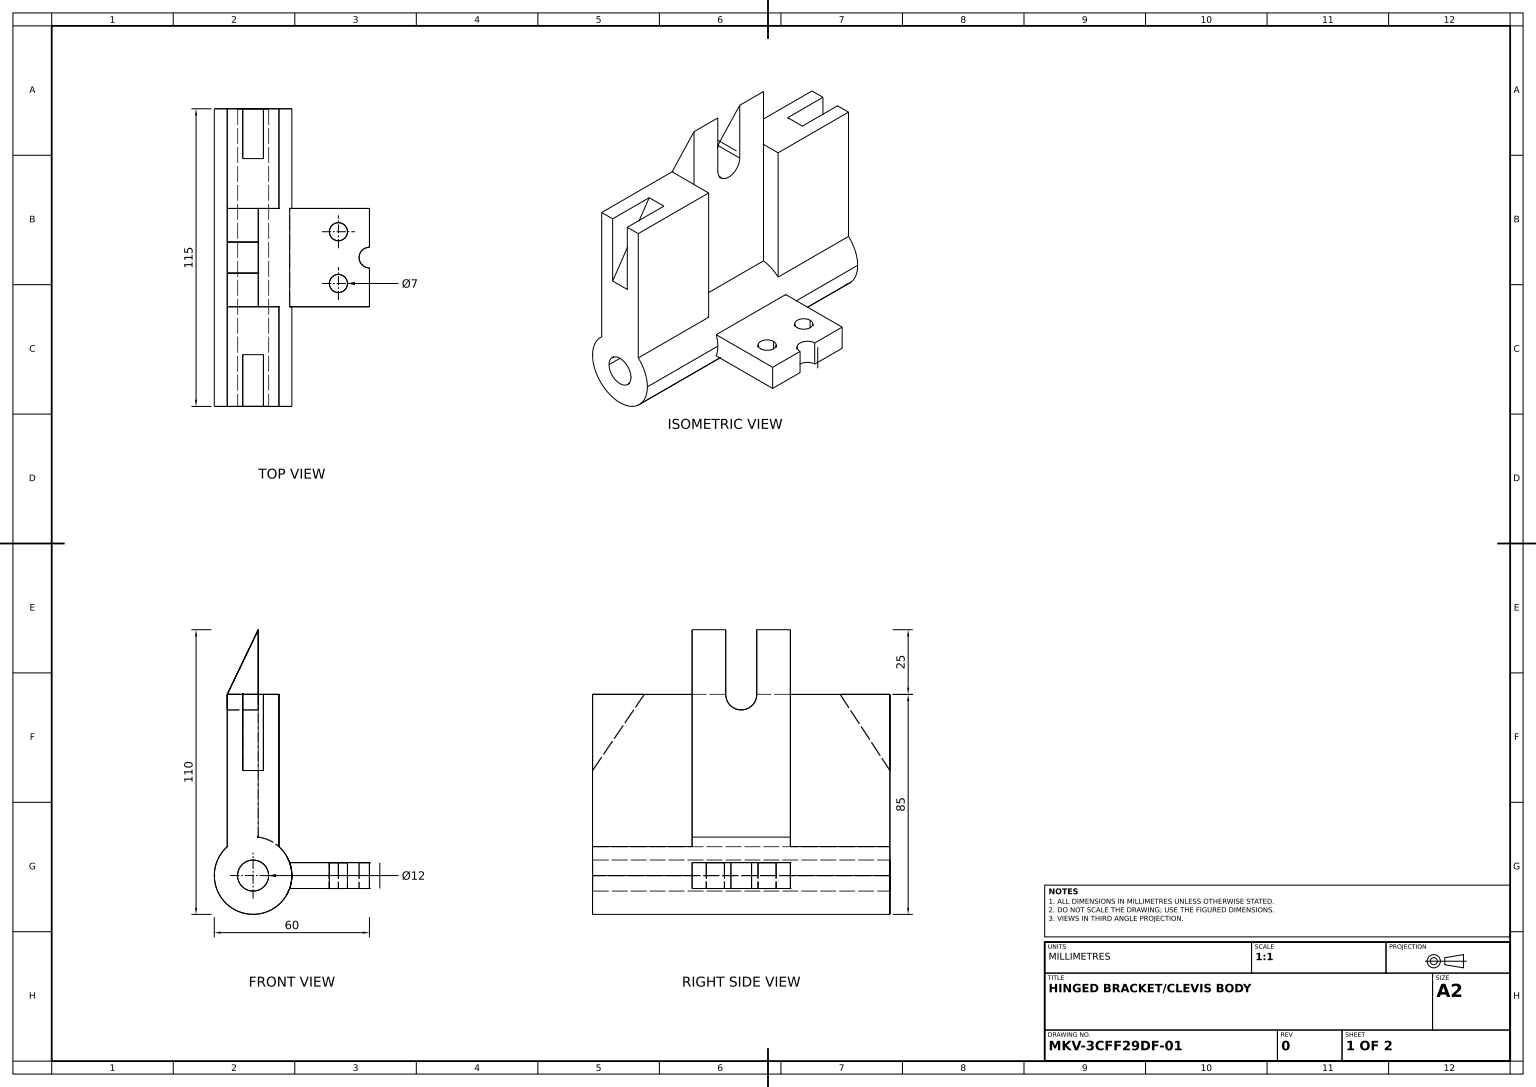
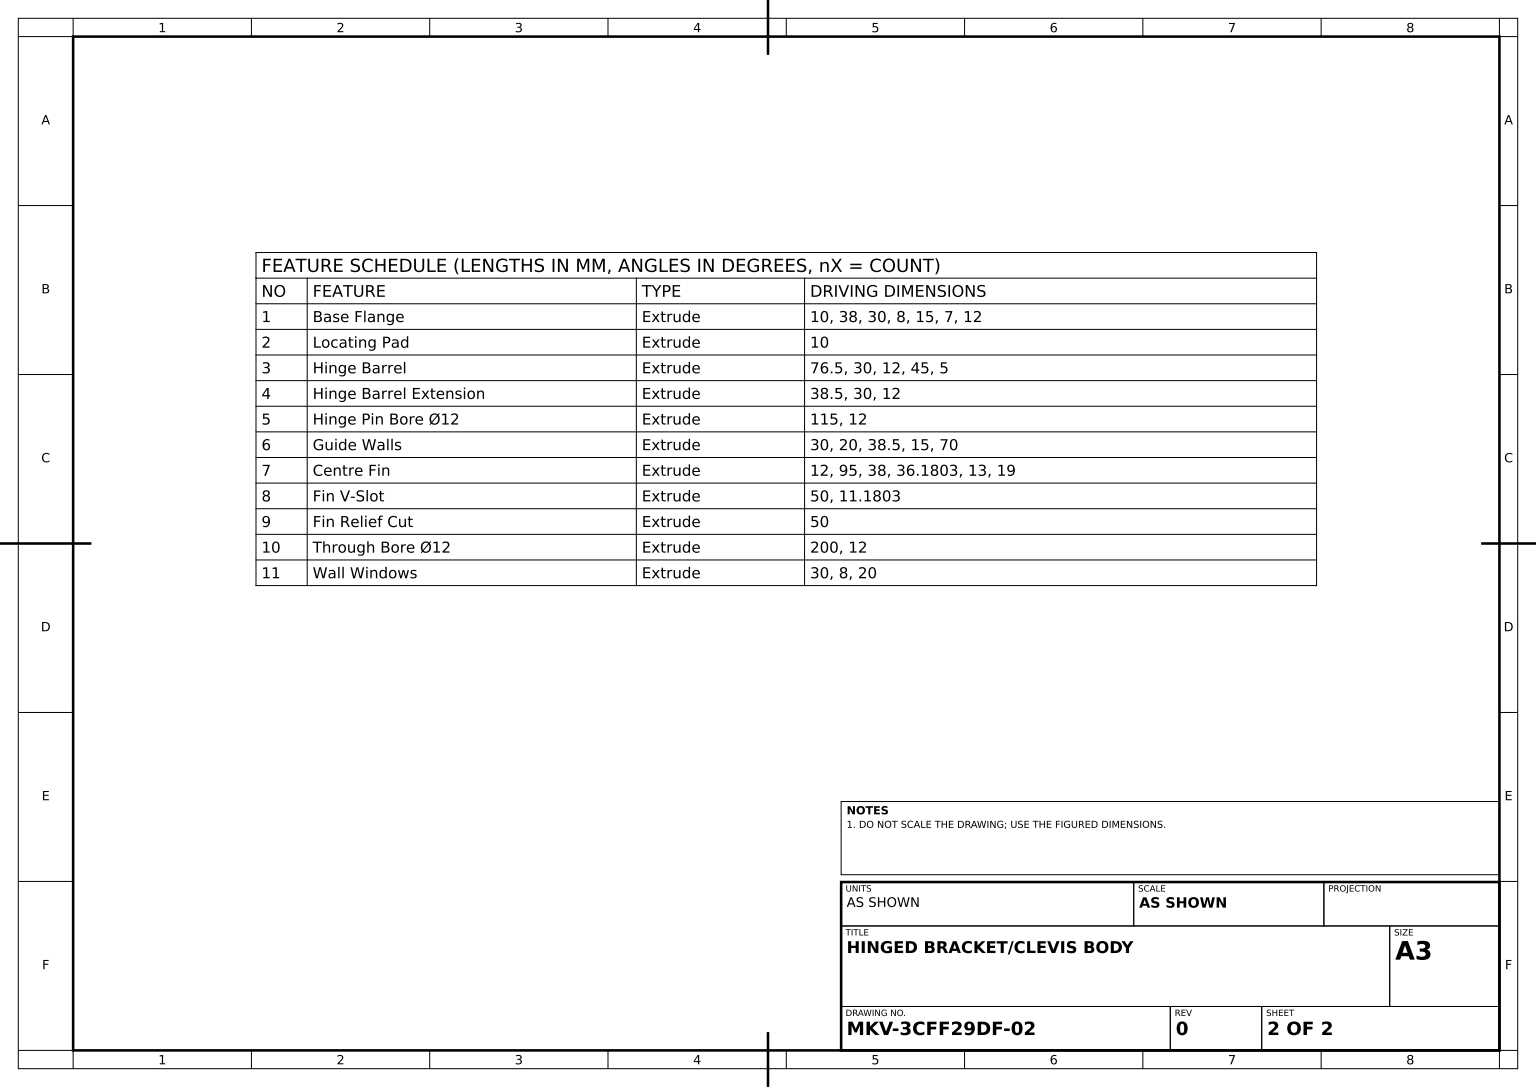
SolidWorks part; units mm, degrees
material "Plain Carbon Steel"
ref_plane "Front Plane" through (0, 0, 0) normal (0, 0, 1) x (1, 0, 0)
ref_plane "Top Plane" through (0, 0, 0) normal (0, 1, 0) x (1, 0, 0)
ref_plane "Right Plane" through (0, 0, 0) normal (1, 0, 0) x (0, 0, -1)
sketch "Base Flange Sketch" plane through (0, 0, 0) normal (0, 1, 0) x (1, 0, 0)
  line L0 (15, -4) -> (15, -19)
  line L1 (-15, 19) -> (15, 19)
  line L2 (-15, 19) -> (-15, -19)
  line L3 (-15, -19) -> (15, -19)
  line L4 (15, 19) -> (15, 4)
  line L5 (-15, 19) -> (15, -19) construction
  line L6 (-15, -19) -> (15, 19) construction
  arc A0 (15, 4) -> (15, -4) centre (15, 0) ccw
  circle A1 centre (3, 10) radius 3.5
  circle A2 centre (3, -10) radius 3.5
  point P0 (0, 0)
  dimension "D3" = 8
  dimension "D6" = 7
  dimension "D7" = 7
  dimension "D1" = 38
  dimension "D2" = 30
  dimension "D4" = 15
  dimension "D5" = 15
  dimension "D8" = 10
  dimension "D9" = 10
  dimension "D10" = 12
  dimension "D11" = 12
extrude "Base Flange" add sketch "Base Flange Sketch" along normal blind 10
sketch "Locating Pad Sketch" plane through (-15, 0, 0) normal (-1, 0, 0) x (0, 0, 1)
  line L1 (-19, 10) -> (19, 10)
  line L2 (-19, 10) -> (-19, 0)
  line L3 (-19, 0) -> (19, 0)
  line L4 (19, 10) -> (19, 0)
extrude "Locating Pad" add sketch "Locating Pad Sketch" along normal blind 10
sketch "Hinge Barrel Sketch" plane through (0, 0, 19) normal (0, 0, 1) x (1, 0, 0)
  line L0 (15, 10) -> (15, 0) construction
  line L1 (-25, 10) -> (15, 10) construction
  circle A0 centre (-30, 5) radius 15
  circle A1 centre (-30, 5) radius 6
  dimension "D1" = 30
  dimension "D2" = 12
  dimension "D3" = 45
  dimension "D4" = 5
extrude "Hinge Barrel" add sketch "Hinge Barrel Sketch" against normal blind 76.5
sketch "Barrel Extension Sketch" plane through (0, 0, 19) normal (0, 0, 1) x (1, 0, 0)
  circle A0 centre (-30, 5) radius 6
  circle A1 centre (-30, 5) radius 15
  dimension "D1" = 30
  dimension "D2" = 12
extrude "Hinge Barrel Extension" add sketch "Barrel Extension Sketch" along normal blind 38.5
sketch "Pin Bore Sketch" plane through (0, 0, 57.5) normal (0, 0, 1) x (1, 0, 0)
  circle A0 centre (-30, 5) radius 6
  dimension "D1" = 12
extrude "Hinge Pin Bore Ø12" cut sketch "Pin Bore Sketch" against normal blind 115
ref_plane "Plane1" through (-30, 0, 0) normal (1, 0, 0) x (0, 0, -1)
sketch "Guide Walls Sketch" plane through (-30, 0, 0) normal (1, 0, 0) x (0, 0, -1)
  line L0 (57.5, 5) -> (19, 5)
  line L1 (57.5, -10) -> (57.5, 20) construction
  line L2 (57.5, 20) -> (-57.5, 20) construction
  line L3 (-57.5, 20) -> (-57.5, -10) construction
  line L4 (57.5, 5) -> (19, 5)
  line L5 (57.5, 5) -> (57.5, 75)
  line L6 (57.5, 75) -> (19, 75)
  line L7 (19, 5) -> (19, 75)
  line L8 (-57.5, 5) -> (-19, 5)
  line L9 (-57.5, 5) -> (-57.5, 75)
  line L10 (-57.5, 75) -> (-19, 75)
  line L11 (-19, 5) -> (-19, 75)
  dimension "D1" = 38.5
  dimension "D2" = 15
  dimension "D3" = 70
  dimension "D4" = 38.5
  dimension "D5" = 70
  dimension "D6" = 38.5
extrude "Guide Walls" add sketch "Guide Walls Sketch" along normal mid plane 20 contours L7 L0 L5 L6 | L8 L11 L10 L9
sketch "Centre Fin Sketch" plane through (-40, 0, 0) normal (-1, 0, 0) x (0, 0, 1)
  line L0 (57.5, 75) -> (19, 75) construction
  line L1 (-19, 16.1803) -> (19, 16.1803)
  line L2 (-19, 16.1803) -> (-19, 111.1803)
  line L3 (-19, 111.1803) -> (-6, 111.1803)
  line L4 (19, 16.1803) -> (19, 111.1803)
  line L6 (6, 75) -> (6, 111.1803)
  line L7 (-6, 75) -> (-6, 111.1803)
  line L8 (6, 111.1803) -> (19, 111.1803)
  arc A0 (-6, 75) -> (6, 75) centre (0, 75) ccw
  point P10 (0, 111.1803)
  dimension "D1" = 95
  dimension "D4" = 12
  dimension "D2" = 38
  dimension "D3" = 0
  dimension "D5" = 36.1803
  dimension "D6" = 36.1803
  dimension "D7" = 13
  dimension "D8" = 19
  dimension "D9" = 13
extrude "Centre Fin" add sketch "Centre Fin Sketch" against normal blind 12
sketch "Fin V-Slot Sketch" plane through (0, 0, 19) normal (0, 0, 1) x (1, 0, 0)
  line L0 (-28, 75) -> (-28, 111.1803) construction
  line L3 (-40, 100) -> (-28, 100)
  line L6 (-40, 111.1803) -> (-28, 111.1803)
  line L7 (-40, 111.1803) -> (-40, 100)
  line L8 (-40, 100) -> (-28, 100)
  line L9 (-28, 111.1803) -> (-28, 100)
  line M2 (-40, 111.1803) -> (-40, 75)
  line M4 (-28, 75) -> (-28, 111.1803)
  line M5 (-28, 111.1803) -> (-40, 111.1803)
  dimension "D1" = 11.1803
extrude "Fin V-Slot" cut sketch "Fin V-Slot Sketch" against normal blind 50 contours L3 M2 M4 M5
sketch "Fin Relief Sketch" plane through (0, 0, 19) normal (0, 0, 1) x (1, 0, 0)
  line L0 (-40, 75) -> (-28, 100)
  line L1 (-28, 100) -> (-40, 100)
  line L2 (-40, 100) -> (-40, 75)
extrude "Fin Relief Cut" cut sketch "Fin Relief Sketch" against normal blind 50
sketch "Through Bore Sketch" plane through (0, 0, 57.5) normal (0, 0, 1) x (1, 0, 0)
  line L0 (-24, 5) -> (-36, 5) construction
  circle A0 centre (-30, 5) radius 6
  dimension "D1" = 12
extrude "Through Bore Ø12" cut sketch "Through Bore Sketch" against normal blind 200
ref_plane "Plane2" through (-30, 0, 0) normal (1, 0, 0) x (0, 0, -1)
sketch "Wall Window Sketch" plane through (-30, 0, 0) normal (1, 0, 0) x (0, 0, -1)
  line L0 (57.5, 75) -> (38.25, 75)
  line L2 (57.5, 75) -> (19, 75) construction
  line L3 (57.5, 75) -> (57.5, 45.5902)
  line L5 (57.5, 16.1803) -> (57.5, 75) construction
  line L6 (57.5, 45.5902) -> (38.25, 75)
  line L7 (-57.5, 75) -> (-57.5, 45.5902)
  line L9 (-57.5, 16.1803) -> (-57.5, 75) construction
  line L10 (-57.5, 45.5902) -> (-37.5, 75)
  line L11 (-57.5, 75) -> (-19, 75) construction
  line L12 (-37.5, 75) -> (-57.5, 75)
  dimension "D1" = 20
extrude "Wall Windows" cut sketch "Wall Window Sketch" against normal mid plane 8
